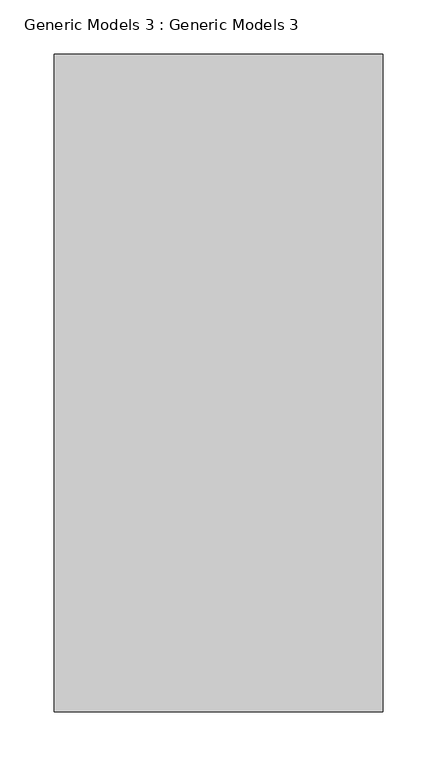
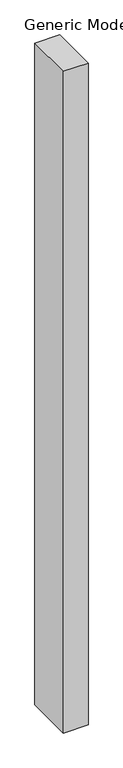
"""IFC4 building model written with IfcOpenShell, lengths in millimetres: proxy geometry, Generic Models 3 : Generic Models 3."""

from ifc_helpers import new_model, si_unit, frame, origin, place, context, project, spatial, polyline, outline, extrude, source, transform, mapped, element, save


def generic_models_3_generic_models_3_72a9eea6(model_context):
    return source(origin(), model_context, "Body", "SweptSolid", [
        extrude(outline(polyline([(-12354.4586008, -8059.5844117), (-12354.4586008, -7449.9844117), (-12049.6586008, -7449.9844117), (-12049.6586008, -8059.5844117), (-12354.4586008, -8059.5844117)])), frame((0.0, 0.0, -15.5768026), z_axis=(0.0, 0.0, 1.0), x_axis=(1.0, 0.0, 0.0)), (0.0, 0.0, 1.0), 8646.4624483),
    ])


if __name__ == "__main__":
    model = new_model("IFC4")
    model_context = context("Model", 3, world=origin())
    ifc_project = project(units=[si_unit("LENGTHUNIT", "METRE", prefix="MILLI")], contexts=[model_context])
    site = spatial("IfcSite", under=ifc_project)
    building = spatial("IfcBuilding", under=site)
    placement = place(None, origin())
    generic_models_3_generic_models_3_shape = generic_models_3_generic_models_3_72a9eea6(model_context)
    element("IfcBuildingElementProxy", 1, Name="Generic Models 3 : Generic Models 3", ObjectType="Generic Models 3 : Generic Models 3", at=placement, inside=building, context=model_context, shape_type="MappedRepresentation", body=[
        mapped(generic_models_3_generic_models_3_shape, transform((0.0, 0.0, 0.0), x_axis=(1.0, 0.0, 0.0), y_axis=(0.0, 1.0, 0.0), z_axis=(0.0, 0.0, 1.0))),
    ])
    save(model, "model.ifc")

# Revit data of these elements
# Element 1 (IfcBuildingElementProxy, "Generic Models 3 : Generic Models 3")
#   Materials on its faces: "ESPRESSO"
# Materials
#   "ESPRESSO": class "Generic", colour RGB 120 120 120, transparency 0, Cost = 0
